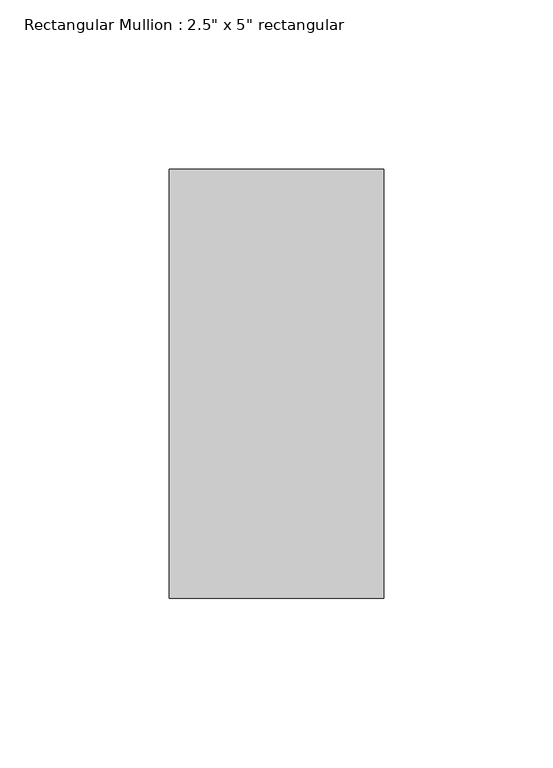
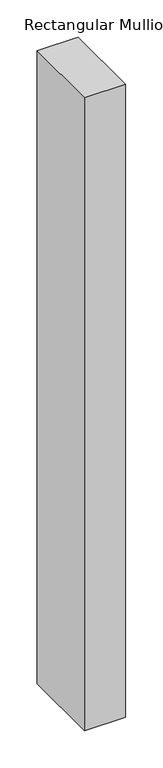
"""IFC4 building model written with IfcOpenShell, lengths in millimetres: member geometry."""

from ifc_helpers import new_model, si_unit, frame, origin, place, context, project, spatial, polyline, outline, extrude, source, transform, mapped, element, save


def member_6ef8dc49(model_context):
    return source(origin(), model_context, "Body", "SweptSolid", [
        extrude(outline(polyline([(0.0, 63.5), (0.0, -63.5), (-63.5, -63.5), (-63.5, 63.5), (0.0, 63.5)])), frame((0.0, 0.0, -1035.05), z_axis=(0.0, 0.0, 1.0), x_axis=(1.0, 0.0, 0.0)), (0.0, 0.0, 1.0), 1035.05),
    ])


if __name__ == "__main__":
    model = new_model("IFC4")
    model_context = context("Model", 3, world=origin())
    ifc_project = project(units=[si_unit("LENGTHUNIT", "METRE", prefix="MILLI")], contexts=[model_context])
    site = spatial("IfcSite", under=ifc_project)
    building = spatial("IfcBuilding", under=site)
    placement = place(None, origin())
    member_shape = member_6ef8dc49(model_context)
    element("IfcMember", 1, ObjectType="Rectangular Mullion : 2.5\" x 5\" rectangular", at=placement, inside=building, context=model_context, shape_type="MappedRepresentation", body=[
        mapped(member_shape, transform((0.0, 0.0, 0.0), x_axis=(1.0, 0.0, 0.0), y_axis=(0.0, 1.0, 0.0), z_axis=(0.0, 0.0, 1.0))),
    ])
    save(model, "model.ifc")

# Revit data of these elements
# Type "Rectangular Mullion : 2.5\" x 5\" rectangular"
#   built-in parameter 1007304 = 0.416667 (stored number, unit not read)
#   built-in parameter 1007301 = 0.104167 (stored number, unit not read)
#   built-in parameter 1007300 = 0.104167 (stored number, unit not read)
# Element 1 (IfcMember, "Rectangular Mullion : 2.5\" x 5\" rectangular")
#   Materials on its faces: "metal black"
# Materials
#   "metal black": class "Generic", colour RGB 120 120 120, transparency 0, Cost = 0
